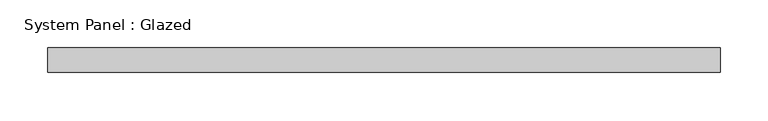
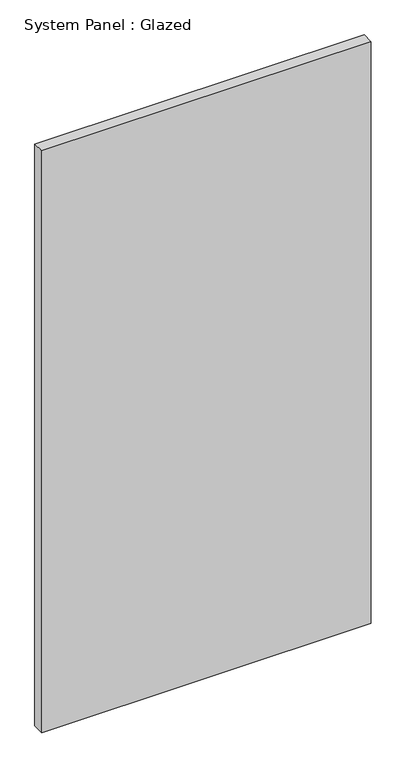
"""IFC4 building model written with IfcOpenShell, lengths in millimetres: plate geometry, System Panel : Glazed."""

from ifc_helpers import new_model, si_unit, origin, origin_with_axes, place, context, project, spatial, polyline, outline, extrude, source, transform, mapped, element, save


def system_panel_glazed_62f7861e(model_context):
    return source(origin(), model_context, "Body", "SweptSolid", [
        extrude(outline(polyline([(350.3083333, 19.05), (-350.3083333, 19.05), (-350.3083333, 44.45), (350.3083333, 44.45), (350.3083333, 19.05)])), origin_with_axes(), (0.0, 0.0, 1.0), 1308.1),
    ])


if __name__ == "__main__":
    model = new_model("IFC4")
    model_context = context("Model", 3, world=origin())
    ifc_project = project(units=[si_unit("LENGTHUNIT", "METRE", prefix="MILLI")], contexts=[model_context])
    site = spatial("IfcSite", under=ifc_project)
    building = spatial("IfcBuilding", under=site)
    placement = place(None, origin())
    system_panel_glazed_shape = system_panel_glazed_62f7861e(model_context)
    element("IfcPlate", 1, ObjectType="System Panel : Glazed", at=placement, inside=building, context=model_context, shape_type="MappedRepresentation", body=[
        mapped(system_panel_glazed_shape, transform((0.0, 0.0, 0.0), x_axis=(1.0, 0.0, 0.0), y_axis=(0.0, 1.0, 0.0), z_axis=(0.0, 0.0, 1.0))),
    ])
    save(model, "model.ifc")

# Revit data of these elements
# Type "System Panel : Glazed"
#   Construction Type Id = "GSP4R"
#   Analytic Construction = "1/8 in Pilkington single glazing"
#   Visual Light Transmittance = 0.9
#   Solar Heat Gain Coefficient = 0.86
#   Heat Transfer Coefficient (U) = 1.18115 BTU/(h·ft²·°F)
# Element 1 (IfcPlate, "System Panel : Glazed")
#   Materials on its faces: "Glass"
# Materials
#   "Glass": class "Glass", colour RGB 0 128 192, transparency 0.75, Description = "Soda Lime Glass", Cost = 0
